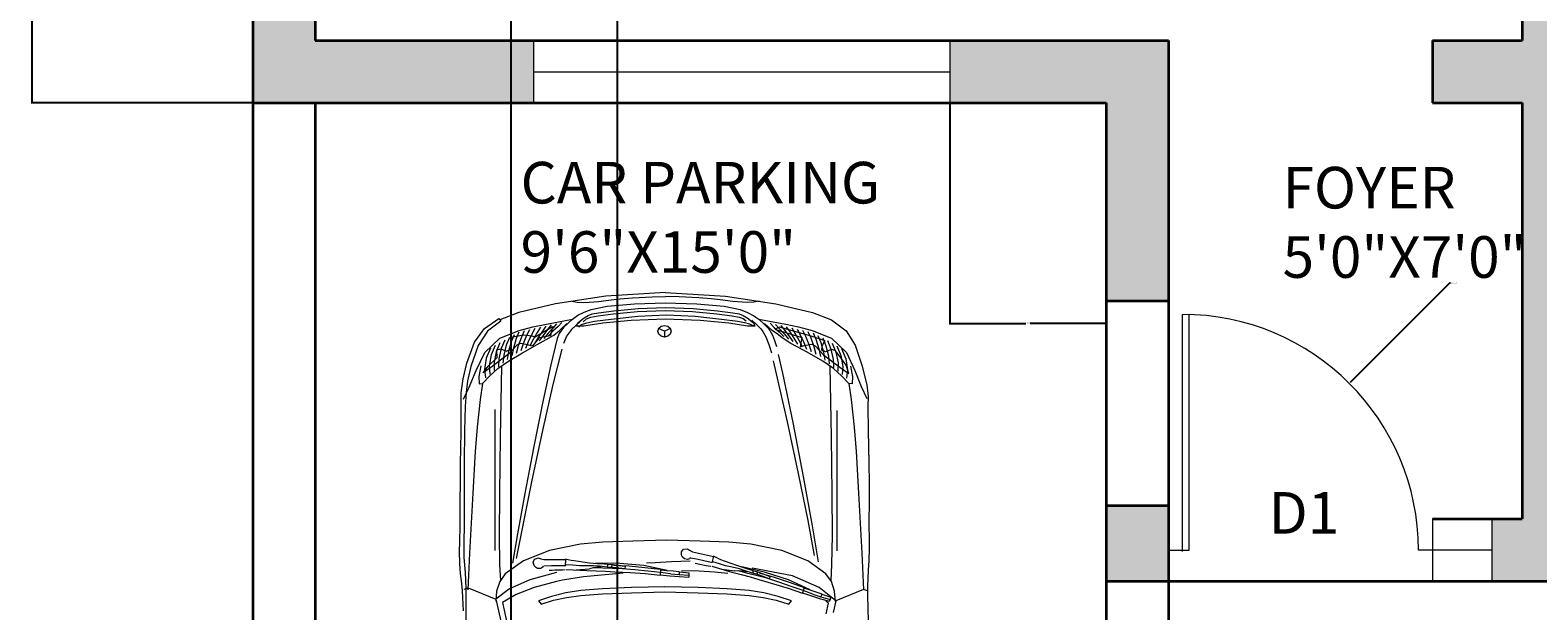
# Model space of a CAD drawing. Units: inches. Extents: x 5 to 421, y -617 to 43.
# Tile 5 of 15: x 5 to 223, y -469 to -385. Entities that reach past the tile are written whole.
import ezdxf

# ---------------------------------------------------------------- set-up
doc = ezdxf.new("R2010")
doc.units = ezdxf.units.IN
doc.header["$MEASUREMENT"] = 0
for name, color, linetype, lineweight in [('A-ANNO-DIMS', 2, 'Continuous', 18), ('A-ANNO-TEXT', 7, 'Continuous', 18), ('A-AREA-IDEN', 7, 'Continuous', 25), ('A-DOOR', 4, 'Continuous', 20), ('A-GLAZ', 4, 'Continuous', 18), ('A-SITE-VEHC', 8, 'Continuous', 13), ('A-WALL', 7, 'Continuous', 35)]:
    doc.layers.add(name, color=color, linetype=linetype, lineweight=lineweight)
doc.layers.add('A-WALL-PATT', color=251, linetype='Continuous', lineweight=13, true_color=0x636466)
doc.styles.get("Standard").update_dxf_attribs({"font": 'arial.ttf'})
doc.dimstyles.get("Standard").update_dxf_attribs({"dimtxt": 0.18, "dimasz": 0.18, "dimexe": 0.18, "dimexo": 0.0625, "dimgap": 0.09, "dimtad": 0, "dimtih": 1, "dimtoh": 1, "dimdec": 0, "dimzin": 0, "dimdsep": 46, "dimlunit": 3, "dimtxsty": 'Standard', "dimcen": 0.09, "dimadec": 0, "dimazin": 0, "dimtfac": 1, "dimtdec": 0, "dimtofl": 0, "dimtmove": 0, "dimatfit": 3, "dimfxl": 1, "dimtolj": 1, "dimtzin": 0, "dimarcsym": 0})

# ---------------------------------------------------------------- blocks, each defined once
blk = doc.blocks.new('WINDOW-W1-60')
for p, q in [((0, 9), (60, 9)), ((0, 0), (0, 9)), ((60, 9), (60, 0)), ((0, 4.5), (60, 4.5)), ((60, 0), (0, 0))]:
    blk.add_line(p, q)
blk = doc.blocks.new('*D55')
at = {"layer": 'A-ANNO-DIMS', "color": 0, "lineweight": -2, "transparency": 16777216}
for p, q in [((370.48, 10.88), (420.4, 10.88)), ((420.22, 10.7), (420.22, -286.69)), ((420.22, -584.44), (420.22, -287.05)), ((169.48, -584.62), (420.4, -584.62))]:
    blk.add_line(p, q, dxfattribs=at)
at = {"layer": 'A-ANNO-DIMS', "color": 0, "transparency": 16777216}
for points in [[(420.19, 10.7), (420.25, 10.7), (420.22, 10.88)], [(420.19, -584.44), (420.25, -584.44), (420.22, -584.62)]]:
    blk.add_solid(points, dxfattribs=at)
at = {"layer": 'Defpoints', "color": 0, "transparency": 16777216}
for p in [(370.42, 10.88), (169.42, -584.62), (420.22, -584.62)]:
    blk.add_point(p, dxfattribs=at)
at = {"layer": 'A-ANNO-DIMS', "color": 0, "transparency": 16777216, "insert": (420.22, -286.87), "char_height": 0.18, "attachment_point": 5}
blk.add_mtext('\\A1;595.5', dxfattribs=at)
blk = doc.blocks.new('*D63')
at = {"layer": 'A-ANNO-DIMS', "color": 0, "lineweight": -2, "transparency": 16777216}
for p, q in [((37.36, -352.8), (5.44, -352.8)), ((5.62, -352.98), (5.62, -374.03)), ((5.62, -395.44), (5.62, -374.39)), ((37.36, -395.62), (5.44, -395.62))]:
    blk.add_line(p, q, dxfattribs=at)
at = {"layer": 'A-ANNO-DIMS', "color": 0, "transparency": 16777216}
for points in [[(5.59, -352.98), (5.65, -352.98), (5.62, -352.8)], [(5.59, -395.44), (5.65, -395.44), (5.62, -395.62)]]:
    blk.add_solid(points, dxfattribs=at)
at = {"layer": 'Defpoints', "color": 0, "transparency": 16777216}
for p in [(37.42, -352.8), (5.62, -395.62), (37.42, -395.62)]:
    blk.add_point(p, dxfattribs=at)
at = {"layer": 'A-ANNO-DIMS', "color": 0, "transparency": 16777216, "insert": (5.62, -374.21), "char_height": 0.18, "attachment_point": 5}
blk.add_mtext('\\A1;42.82', dxfattribs=at)
blk = doc.blocks.new('*D74')
at = {"layer": 'A-ANNO-DIMS', "color": 0, "lineweight": -2, "transparency": 16777216}
for p, q in [((137.92, -395.68), (137.92, -427.6)), ((160.42, -395.68), (160.42, -427.6)), ((138.1, -427.42), (148.84, -427.42)), ((160.24, -427.42), (149.5, -427.42))]:
    blk.add_line(p, q, dxfattribs=at)
at = {"layer": 'A-ANNO-DIMS', "color": 0, "transparency": 16777216}
for points in [[(138.1, -427.39), (138.1, -427.45), (137.92, -427.42)], [(160.24, -427.39), (160.24, -427.45), (160.42, -427.42)]]:
    blk.add_solid(points, dxfattribs=at)
at = {"layer": 'Defpoints', "color": 0, "transparency": 16777216}
for p in [(137.92, -395.62), (160.42, -395.62), (137.92, -427.42)]:
    blk.add_point(p, dxfattribs=at)
at = {"layer": 'A-ANNO-DIMS', "color": 0, "transparency": 16777216, "insert": (149.17, -427.42), "char_height": 0.18, "attachment_point": 5}
blk.add_mtext('\\A1;22.5', dxfattribs=at)
blk = doc.blocks.new('*D78')
at = {"layer": 'A-ANNO-DIMS', "color": 0, "lineweight": -2, "transparency": 16777216}
for p, q in [((74.62, -338.19), (74.62, -616.6)), ((89.92, -338.33), (89.92, -616.6)), ((74.8, -616.42), (81.96, -616.42)), ((89.74, -616.42), (82.59, -616.42))]:
    blk.add_line(p, q, dxfattribs=at)
at = {"layer": 'A-ANNO-DIMS', "color": 0, "transparency": 16777216}
for points in [[(74.8, -616.39), (74.8, -616.45), (74.62, -616.42)], [(89.74, -616.39), (89.74, -616.45), (89.92, -616.42)]]:
    blk.add_solid(points, dxfattribs=at)
at = {"layer": 'Defpoints', "color": 0, "transparency": 16777216}
for p in [(74.62, -338.13), (89.92, -338.27), (89.92, -616.42)]:
    blk.add_point(p, dxfattribs=at)
at = {"layer": 'A-ANNO-DIMS', "color": 0, "transparency": 16777216, "insert": (82.27, -616.42), "char_height": 0.18, "attachment_point": 5}
blk.add_mtext('\\A1;15.3', dxfattribs=at)
blk = doc.blocks.new('*D80')
at = {"layer": 'A-ANNO-DIMS', "color": 0, "lineweight": -2, "transparency": 16777216}
for p, q in [((209.91, -421.62), (195.6, -435.95)), ((210.09, -421.62), (209.91, -421.62)), ((171.33, -460.16), (171.51, -460.16)), ((171.42, -460.25), (171.42, -460.07))]:
    blk.add_line(p, q, dxfattribs=at)
at = {"layer": 'A-ANNO-DIMS', "color": 0, "transparency": 16777216}
blk.add_solid([(195.58, -435.93), (195.63, -435.97), (195.48, -436.07)], dxfattribs=at)
at = {"layer": 'Defpoints', "color": 0, "transparency": 16777216}
for p in [(195.48, -436.07), (171.42, -460.16)]:
    blk.add_point(p, dxfattribs=at)
at = {"layer": 'A-ANNO-DIMS', "color": 0, "transparency": 16777216, "insert": (210.64, -421.62), "char_height": 0.18, "attachment_point": 5}
blk.add_mtext('\\A1;R34.045', dxfattribs=at)

msp = doc.modelspace()

# ---------------------------------------------------------------- hatches: boundary and pattern name
at = {"layer": 'A-WALL-PATT'}
h = msp.add_hatch(color=256, dxfattribs=at)
h.dxf.hatch_style = 1
h.paths.add_polyline_path([(46.4196, -88.1188), (37.4196, -88.1188), (37.4196, -166.6119), (46.4196, -166.6119), (46.4196, -122.6188), (135.4196, -122.6188), (135.4196, -120.3688), (135.4196, -118.1188), (46.4196, -118.1188)])
h.paths.add_polyline_path([(82.4196, 10.8812), (37.4196, 10.8812), (37.4196, -28.1188), (46.4196, -28.1188), (46.4196, 1.8812), (82.4196, 1.8812)])
h.paths.add_polyline_path([(215.5968, 10.8812), (142.4196, 10.8812), (142.4196, 1.8812), (178.4196, 1.8812), (178.4196, -118.1188), (175.4196, -118.1188), (175.4196, -122.6188), (182.9196, -122.6188), (182.9196, -80.6188), (211.9196, -80.6188), (211.9196, -78.3688), (211.9196, -76.1188), (182.9196, -76.1188), (182.9196, 1.8812), (215.5968, 1.8812)])
h.paths.add_polyline_path([(274.4196, 10.8812), (239.5968, 10.8812), (239.5968, 1.8812), (242.9196, 1.8812), (242.9196, -76.1188), (239.9196, -76.1188), (239.9196, -80.6188), (242.9196, -80.6188), (242.9196, -83.6188), (247.4196, -83.6188), (247.4196, 1.8812), (274.4196, 1.8812)])
h.paths.add_polyline_path([(370.4196, 10.8812), (334.4196, 10.8812), (334.4196, 1.8812), (361.4196, 1.8812), (361.4196, -28.1188), (370.4196, -28.1188)])
h.paths.add_polyline_path([(370.4196, -88.1188), (361.4196, -88.1188), (361.4196, -118.1188), (247.4196, -118.1188), (247.4196, -115.1188), (242.9196, -115.1188), (242.9196, -118.1188), (220.4196, -118.1188), (220.4196, -158.6188), (224.9196, -158.6188), (224.9196, -122.6188), (326.9196, -122.6188), (326.9196, -170.7662), (331.4196, -170.7662), (331.4196, -122.6188), (370.4196, -122.6188)])
h.paths.add_polyline_path([(388.4196, -122.6188), (388.4196, -118.1188), (379.4196, -118.1188), (379.4196, -122.6188), (379.4196, -154.8688), (388.4196, -154.8688)])
h.paths.add_polyline_path([(388.4196, -214.8688), (379.4196, -214.8688), (379.4196, -247.1188), (388.4196, -247.1188)])
h.paths.add_polyline_path([(371.0265, -242.6188), (331.4196, -242.6188), (331.4196, -239.6188), (326.9196, -239.6188), (326.9196, -242.6188), (224.9196, -242.6188), (224.9196, -206.6188), (220.4196, -206.6188), (220.4196, -343.6188), (224.9196, -343.6188), (229.4196, -343.6188), (229.4196, -247.1188), (261.5265, -247.1188), (261.5265, -276.1188), (263.7765, -276.1188), (266.0265, -276.1188), (266.0265, -247.1188), (362.0265, -247.1188), (362.0265, -265.1188), (371.0265, -265.1188), (371.0265, -247.1188)])
h.paths.add_polyline_path([(371.0265, -289.1188), (362.0265, -289.1188), (362.0265, -307.1188), (266.0265, -307.1188), (266.0265, -304.1188), (261.5265, -304.1188), (261.5265, -307.1188), (261.5265, -311.6188), (362.0265, -311.6188), (362.0265, -353.6188), (371.0265, -353.6188)])
h.paths.add_polyline_path([(371.0265, -413.6188), (362.0265, -413.6188), (362.0265, -455.6188), (325.7231, -455.6188), (325.7231, -464.6188), (361.4196, -464.6188), (371.0265, -464.6188)])
h.paths.add_polyline_path([(265.7231, -455.6188), (229.4196, -455.6188), (229.4196, -383.6188), (220.4196, -383.6188), (220.4196, -386.6188), (207.4649, -386.6188), (207.4649, -395.6188), (220.4196, -395.6188), (220.4196, -455.6188), (216.0568, -455.6188), (216.0568, -464.6188), (265.7231, -464.6188)])
h.paths.add_polyline_path([(169.4196, -386.6188), (137.9196, -386.6188), (137.9196, -395.6188), (160.4196, -395.6188), (160.4196, -424.2032), (169.4196, -424.2032)])
h.paths.add_polyline_path([(169.4196, -453.7423), (160.4196, -453.7423), (160.4196, -464.6188), (169.4196, -464.6188)])
h.paths.add_polyline_path([(46.4196, -575.6188), (37.4196, -575.6188), (37.4196, -584.6188), (46.4196, -584.6188)])
h.paths.add_polyline_path([(169.4196, -575.6188), (160.4196, -575.6188), (160.4196, -579.5504), (160.4196, -584.6188), (169.4196, -584.6188)])
h.paths.add_polyline_path([(46.4196, -226.6119), (37.4196, -226.6119), (37.4196, -292.8008), (46.4196, -292.8008)])
h.paths.add_polyline_path([(46.4196, -352.8008), (37.4196, -352.8008), (37.4196, -395.6188), (77.9196, -395.6188), (77.9196, -386.6188), (46.4196, -386.6188)])

# ---------------------------------------------------------------- linework, layer by layer
at = {"layer": 'A-DOOR'}
for p, q in [((171.4196, -460.1188), (171.4196, -426.1188)), ((172.4196, -460.1188), (172.4196, -426.1188)), ((207.4649, -455.6188), (207.4649, -464.6188)), ((169.4196, -460.1188), (172.4196, -460.1188)), ((207.4649, -460.1188), (205.4649, -460.1188))]:
    msp.add_line(p, q, dxfattribs=at)
msp.add_arc((171.4196, -460.1641), 34.0453, 0.076254, 90, dxfattribs=at)
at = {"layer": 'A-GLAZ'}
for p, q in [((216.0568, -455.6188), (216.0568, -464.6188)), ((216.0568, -460.1188), (207.4649, -460.1188))]:
    msp.add_line(p, q, dxfattribs=at)
at = {"layer": 'A-SITE-VEHC'}
for p, q in [((88.2888, -423.4807), (81.054, -424.5837)), ((96.9277, -422.9659), (88.2888, -423.4807)), ((90.3721, -423.8704), (92.147, -423.7322)), ((92.147, -423.7322), (94.9644, -423.5941)), ((94.9644, -423.5941), (96.9277, -423.5314)), ((96.9277, -422.9659), (105.5667, -423.4807)), ((98.8913, -423.5941), (96.9277, -423.5314)), ((101.7086, -423.7322), (98.8913, -423.5941)), ((103.4836, -423.8704), (101.7086, -423.7322)), ((105.5667, -423.4807), (112.8017, -424.5837)), ((75.7796, -425.8668), (73.0219, -426.9221)), ((81.054, -424.5837), (75.7796, -425.8668)), ((83.4206, -424.2094), (84.1909, -424.3664)), ((84.1909, -424.3664), (85.0994, -424.4103)), ((84.2586, -426.238), (85.1677, -425.8108)), ((85.0994, -424.4103), (85.9073, -424.3788)), ((85.1677, -425.8108), (86.19, -425.3963)), ((85.9073, -424.3788), (87.228, -424.2471)), ((86.19, -425.3963), (88.484, -424.9461)), ((86.3168, -426.0614), (87.2637, -425.9046)), ((87.228, -424.2471), (89.0889, -424.0399)), ((87.2637, -425.9046), (89.4679, -425.6243)), ((88.484, -424.9461), (92.4484, -424.584)), ((89.0889, -424.0399), (90.3721, -423.8704)), ((89.3807, -426.0595), (92.8658, -425.7162)), ((89.4679, -425.6243), (92.9529, -425.281)), ((92.4484, -424.584), (96.9277, -424.4355)), ((92.8658, -425.7162), (96.8408, -425.5487)), ((92.9529, -425.281), (96.9277, -425.1136)), ((96.8408, -425.5487), (100.8158, -425.7162)), ((96.9277, -424.4355), (101.4072, -424.584)), ((96.9277, -425.1136), (100.9027, -425.281)), ((100.8158, -425.7162), (104.3009, -426.0595)), ((100.9027, -425.281), (104.3878, -425.6243)), ((101.4072, -424.584), (105.3717, -424.9461)), ((104.7667, -424.0399), (103.4836, -423.8704)), ((104.3878, -425.6243), (106.592, -425.9046)), ((106.6275, -424.2471), (104.7667, -424.0399)), ((105.3717, -424.9461), (107.6657, -425.3963)), ((106.592, -425.9046), (107.5389, -426.0614)), ((107.9481, -424.3788), (106.6275, -424.2471)), ((107.6657, -425.3963), (108.7179, -425.8544)), ((108.7562, -424.4103), (107.9481, -424.3788)), ((108.7179, -425.8544), (109.6569, -426.325)), ((109.6648, -424.3664), (108.7562, -424.4103)), ((110.4351, -424.2094), (109.6648, -424.3664)), ((112.8017, -424.5837), (118.0761, -425.8668)), ((118.0761, -425.8668), (120.8338, -426.9221)), ((69.3711, -430.1379), (70.8148, -428.1461)), ((70.8148, -428.1461), (72.9016, -426.7215)), ((73.177, -427.1185), (71.256, -428.5348)), ((72.9016, -426.7215), (73.177, -427.1185)), ((75.7932, -428.4396), (77.7692, -427.9392)), ((78.0926, -428.1602), (77.642, -428.9679)), ((77.7692, -427.9392), (79.7514, -427.5207)), ((78.0971, -429.3429), (80.6258, -427.874)), ((78.8694, -427.9893), (78.4005, -428.7497)), ((79.6462, -427.8179), (79.1591, -428.5313)), ((79.7514, -427.5207), (82.2485, -427.0394)), ((80.4227, -427.6467), (79.9176, -428.313)), ((80.6762, -428.0946), (79.9739, -428.8381)), ((80.6258, -427.874), (80.3167, -429.2124)), ((81.1994, -427.4754), (80.6762, -428.0946)), ((81.4347, -427.8765), (80.6882, -428.5311)), ((81.9759, -427.3041), (81.4347, -427.8765)), ((82.2242, -428.0064), (81.591, -428.8858)), ((81.6239, -428.4674), (82.6858, -427.4308)), ((83.4772, -426.8091), (82.2242, -428.0064)), ((82.2485, -427.0394), (83.4772, -426.8091)), ((84.6587, -427.1007), (83.3473, -428.2992)), ((83.4772, -426.8091), (84.2586, -426.238)), ((84.0633, -427.8201), (84.2663, -427.324)), ((85.1161, -427.8262), (84.0633, -427.8201)), ((84.2663, -427.324), (85.1728, -426.6394)), ((84.4199, -427.9596), (84.8137, -427.5957)), ((84.8137, -427.5957), (85.5658, -427.3175)), ((85.0283, -427.1794), (85.4994, -426.7674)), ((87.8536, -427.4118), (85.1161, -427.8262)), ((85.1728, -426.6394), (85.7717, -426.2683)), ((85.4994, -426.7674), (86.1435, -426.5169)), ((85.5658, -427.3175), (86.6818, -427.1141)), ((85.7717, -426.2683), (86.3168, -426.0614)), ((86.1435, -426.5169), (87.1768, -426.3398)), ((86.6818, -427.1141), (89.0706, -426.8021)), ((87.1768, -426.3398), (89.3807, -426.0595)), ((91.9601, -426.9974), (87.8536, -427.4118)), ((89.0706, -426.8021), (92.8988, -426.4005)), ((96.8713, -426.8091), (91.9601, -426.9974)), ((92.8988, -426.4005), (97.0582, -426.2017)), ((95.8093, -428.5451), (95.9396, -428.1204)), ((96.7635, -428.5451), (95.908, -428.1803)), ((95.9396, -428.1204), (96.2818, -427.8187)), ((96.2818, -427.8187), (96.7635, -427.704)), ((96.7635, -427.704), (97.2447, -427.8187)), ((97.6185, -428.1803), (96.7635, -428.5451)), ((101.9075, -426.9974), (96.8713, -426.8091)), ((97.0582, -426.2017), (101.1968, -426.4005)), ((97.2447, -427.8187), (97.587, -428.1204)), ((97.587, -428.1204), (97.7172, -428.5451)), ((101.1968, -426.4005), (104.9857, -426.8021)), ((106.0206, -427.4118), (101.9075, -426.9974)), ((104.3009, -426.0595), (106.505, -426.3398)), ((104.9857, -426.8021), (107.3534, -427.1141)), ((108.7396, -427.8262), (106.0206, -427.4118)), ((106.505, -426.3398), (107.5061, -426.5108)), ((107.3534, -427.1141), (108.3197, -427.2686)), ((107.5061, -426.5108), (108.1116, -426.7281)), ((107.5389, -426.0614), (108.084, -426.2683)), ((108.084, -426.2683), (108.6829, -426.6394)), ((108.1116, -426.7281), (108.5549, -427.0488)), ((108.3197, -427.2686), (108.9991, -427.4664)), ((108.6829, -426.6394), (109.5893, -427.324)), ((109.7923, -427.8201), (108.7396, -427.8262)), ((108.9991, -427.4664), (109.5727, -427.767)), ((109.3336, -426.9632), (110.1205, -427.6759)), ((109.5893, -427.324), (109.7923, -427.8201)), ((109.6569, -426.325), (110.3785, -426.8091)), ((110.1205, -427.6759), (110.6529, -428.1921)), ((110.3785, -426.8091), (111.1529, -427.5355)), ((110.3785, -426.8091), (111.9209, -427.0823)), ((110.6529, -428.1921), (110.9445, -428.5744)), ((111.1529, -427.5355), (111.6762, -428.0607)), ((112.3063, -428.4628), (111.1699, -427.4308)), ((111.6762, -428.0607), (111.9609, -428.448)), ((111.9209, -427.0823), (114.2611, -427.5423)), ((111.9928, -427.3914), (112.5341, -427.9635)), ((112.5341, -427.9635), (113.2805, -428.6182)), ((113.3429, -427.9612), (112.6534, -428.2674)), ((112.7696, -427.5623), (113.2927, -428.1817)), ((113.2927, -428.1817), (113.9949, -428.9252)), ((116.2301, -428.8039), (113.3429, -427.9612)), ((113.5461, -427.7336), (114.0511, -428.4001)), ((114.2611, -427.5423), (116.0865, -427.9392)), ((114.3225, -427.9048), (114.8095, -428.6184)), ((115.0993, -428.0761), (115.5682, -428.8366)), ((116.0865, -427.9392), (118.0625, -428.4396)), ((120.8338, -426.9221), (122.9445, -428.4988)), ((68.2734, -433.1631), (69.3711, -430.1379)), ((71.256, -428.5348), (69.9184, -430.6081)), ((70.8743, -431.6128), (73.0385, -429.5678)), ((73.0423, -430.2084), (72.5012, -431.5059)), ((73.0385, -429.5678), (75.7932, -428.4396)), ((73.7226, -429.8248), (73.2176, -431.0352)), ((74.4026, -429.4412), (73.9338, -430.5644)), ((74.65, -430.0936), (74.2772, -431.4987)), ((74.6156, -429.4297), (76.4147, -429.0668)), ((74.639, -429.7757), (74.6156, -429.4297)), ((74.6409, -430.5092), (74.639, -429.7757)), ((75.0826, -429.0576), (74.65, -430.0936)), ((75.3663, -429.6228), (74.9727, -430.9883)), ((75.7626, -428.674), (75.3663, -429.6228)), ((75.9564, -430.3259), (75.464, -430.557)), ((76.1248, -429.4047), (75.6872, -430.6813)), ((77.0534, -430.5351), (75.9564, -430.3259)), ((76.539, -428.5027), (76.1248, -429.4047)), ((76.8835, -429.1863), (76.4017, -430.3741)), ((76.4147, -429.0668), (77.6427, -429.1952)), ((77.1161, -430.0668), (76.71, -431.0374)), ((77.3162, -428.3315), (76.8835, -429.1863)), ((77.642, -428.9679), (77.1161, -430.0668)), ((77.8305, -429.7597), (77.3697, -430.6786)), ((77.6427, -429.1952), (78.0971, -429.3429)), ((78.7064, -429.517), (77.6619, -430.7102)), ((78.4005, -428.7497), (77.8305, -429.7597)), ((78.5449, -429.4525), (78.0296, -430.3192)), ((78.4145, -430.4721), (80.1428, -429.5218)), ((79.1591, -428.5313), (78.5449, -429.4525)), ((79.2594, -429.1454), (78.6892, -429.9604)), ((80.3167, -429.2124), (78.7064, -429.517)), ((79.9176, -428.313), (79.2594, -429.1454)), ((79.9739, -428.8381), (79.3491, -429.6011)), ((80.6882, -428.5311), (80.0088, -429.2423)), ((80.1428, -429.5218), (80.8255, -429.102)), ((81.3112, -429.596), (80.3544, -433.4005)), ((80.8255, -429.102), (81.6239, -428.4674)), ((81.591, -428.8858), (81.3112, -429.596)), ((82.3299, -429.9862), (82.2169, -430.333)), ((82.6517, -429.2407), (82.3299, -429.9862)), ((83.3473, -428.2992), (82.6517, -429.2407)), ((95.9396, -428.9696), (95.8093, -428.5451)), ((96.2818, -429.2716), (95.9396, -428.9696)), ((96.7635, -429.3865), (96.2818, -429.2716)), ((96.7635, -428.5451), (96.7635, -429.3865)), ((97.2447, -429.2716), (96.7635, -429.3865)), ((97.587, -428.9696), (97.2447, -429.2716)), ((97.7172, -428.5451), (97.587, -428.9696)), ((110.9445, -428.5744), (111.3801, -429.3839)), ((111.3801, -429.3839), (111.8254, -430.4731)), ((111.9609, -428.448), (112.3202, -429.1271)), ((113.1791, -429.0928), (112.3063, -428.4628)), ((112.3202, -429.1271), (112.6292, -429.9037)), ((112.6292, -429.9037), (112.8982, -430.7589)), ((112.6534, -428.2674), (116.5621, -429.4677)), ((113.7129, -429.5218), (113.1791, -429.0928)), ((113.2805, -428.6182), (113.9599, -429.3291)), ((114.9855, -430.311), (113.7129, -429.5218)), ((113.9949, -428.9252), (114.6195, -429.6882)), ((114.0511, -428.4001), (114.7092, -429.2325)), ((114.7092, -429.2325), (115.2792, -430.0474)), ((114.8095, -428.6184), (115.4237, -429.5396)), ((117.3382, -431.5773), (114.9855, -430.311)), ((115.4237, -429.5396), (115.9391, -430.4065)), ((115.5682, -428.8366), (116.1383, -429.8467)), ((115.8761, -428.2474), (116.3267, -429.055)), ((116.1383, -429.8467), (116.5991, -430.7656)), ((116.7357, -428.9249), (116.2301, -428.8039)), ((116.5621, -429.4677), (116.3069, -430.7974)), ((116.3267, -429.055), (116.8525, -430.1539)), ((116.6525, -428.4187), (117.0852, -429.2733)), ((118.0587, -429.2957), (116.7357, -428.9249)), ((116.8525, -430.1539), (117.2587, -431.1247)), ((117.0852, -429.2733), (117.5669, -430.461)), ((117.4293, -428.59), (117.8439, -429.4917)), ((117.8439, -429.4917), (118.2815, -430.7682)), ((119.909, -429.9274), (118.0587, -429.2957)), ((118.0625, -428.4396), (120.8172, -429.5678)), ((118.2061, -428.7609), (118.6025, -429.7099)), ((118.6025, -429.7099), (118.996, -431.0754)), ((118.8861, -429.1445), (119.3186, -430.1807)), ((119.3186, -430.1807), (119.6916, -431.5858)), ((119.4719, -430.7027), (119.7415, -430.1668)), ((119.5662, -429.5281), (120.0349, -430.6515)), ((119.7415, -430.1668), (119.909, -429.9274)), ((120.2461, -429.9118), (120.751, -431.1223)), ((120.8172, -429.5678), (122.9814, -431.6128)), ((120.9262, -430.2954), (121.4674, -431.5931)), ((122.9445, -428.4988), (124.2439, -430.5614)), ((69.9184, -430.6081), (68.8652, -433.6607)), ((69.6163, -434.2354), (70.8743, -431.6128)), ((71.0689, -432.4475), (70.7995, -434.0515)), ((71.6826, -430.9754), (71.0689, -432.4475)), ((71.3212, -433.5838), (72.65, -432.3556)), ((71.7852, -431.9768), (71.495, -433.541)), ((72.3626, -430.592), (71.7852, -431.9768)), ((74.2891, -431.8677), (71.9248, -433.6635)), ((72.5012, -431.5059), (72.1905, -433.0304)), ((72.608, -431.2511), (73.1494, -431.1126)), ((72.65, -432.3556), (72.608, -431.2511)), ((72.8862, -432.5199), (72.8414, -433.683)), ((73.2176, -431.0352), (72.8862, -432.5199)), ((73.1494, -431.1126), (73.9886, -431.4394)), ((73.5817, -432.0093), (73.4711, -433.1602)), ((73.9338, -430.5644), (73.5817, -432.0093)), ((73.9886, -431.4394), (74.5191, -431.174)), ((74.2772, -431.4987), (74.1008, -432.6375)), ((74.265, -432.8562), (76.2895, -431.658)), ((75.464, -430.557), (74.2891, -431.8677)), ((74.5191, -431.174), (74.6409, -430.5092)), ((74.9727, -430.9883), (74.7305, -432.1151)), ((75.6872, -430.6813), (75.3905, -431.756)), ((76.4017, -430.3741), (76.0504, -431.3969)), ((76.2895, -431.658), (78.4145, -430.4721)), ((77.6619, -430.7102), (77.0534, -430.5351)), ((81.9727, -431.1396), (80.6692, -436.2199)), ((111.8254, -430.4731), (112.1838, -431.6837)), ((113.1414, -431.9011), (113.3375, -432.7409)), ((116.3069, -430.7974), (116.9153, -430.6223)), ((116.9153, -430.6223), (118.0123, -430.4132)), ((119.5903, -432.8562), (117.3382, -431.5773)), ((117.5669, -430.461), (117.9184, -431.4838)), ((118.0123, -430.4132), (118.5048, -430.6443)), ((118.2815, -430.7682), (118.5783, -431.8429)), ((118.5048, -430.6443), (119.6796, -431.9549)), ((118.996, -431.0754), (119.2379, -432.202)), ((119.4496, -431.2613), (119.4719, -430.7027)), ((119.9802, -431.5265), (119.4496, -431.2613)), ((119.6796, -431.9549), (122.0438, -433.7505)), ((119.6916, -431.5858), (119.8679, -432.7248)), ((120.8193, -431.1998), (119.9802, -431.5265)), ((120.0349, -430.6515), (120.3871, -432.0964)), ((120.3871, -432.0964), (120.4976, -433.2471)), ((120.751, -431.1223), (121.0826, -432.607)), ((121.3607, -431.3383), (120.8193, -431.1998)), ((121.9401, -432.0338), (121.3607, -431.3383)), ((121.4674, -431.5931), (121.7781, -433.1176)), ((121.6061, -430.679), (122.1836, -432.0637)), ((122.9582, -433.4664), (121.9401, -432.0338)), ((122.1836, -432.0637), (122.4737, -433.628)), ((122.2864, -431.0626), (122.8999, -432.5347)), ((122.8999, -432.5347), (123.1693, -434.1386)), ((122.9814, -431.6128), (124.2013, -434.2101)), ((124.2439, -430.5614), (125.2421, -433.591)), ((67.7369, -435.4045), (68.2734, -433.1631)), ((68.8652, -433.6607), (68.3838, -435.6874)), ((68.6094, -436.6196), (69.6163, -434.2354)), ((70.2847, -433.5477), (69.979, -435.0678)), ((70.6339, -434.568), (71.3212, -433.5838)), ((71.9248, -433.6635), (70.6339, -434.568)), ((70.7995, -434.0515), (70.952, -435.2509)), ((71.495, -433.541), (71.5816, -434.7281)), ((71.5776, -434.9912), (72.733, -433.9426)), ((72.1905, -433.0304), (72.2117, -434.2057)), ((72.733, -433.9426), (74.265, -432.8562)), ((73.248, -433.591), (73.0571, -443.8216)), ((80.3544, -433.4005), (79.1612, -438.9485)), ((112.4369, -432.8317), (112.5824, -433.454)), ((112.5824, -433.454), (112.7269, -434.0792)), ((112.7269, -434.0792), (112.8734, -434.7023)), ((112.8734, -434.7023), (114.4492, -441.6229)), ((113.3375, -432.7409), (113.5855, -433.768)), ((113.5855, -433.768), (113.7826, -434.6088)), ((113.7826, -434.6088), (115.2521, -441.7013)), ((121.1226, -433.9426), (119.5903, -432.8562)), ((120.6077, -433.591), (120.7986, -443.8216)), ((121.0826, -432.607), (121.1273, -433.7699)), ((122.278, -434.9912), (121.1226, -433.9426)), ((121.7781, -433.1176), (121.7573, -434.2926)), ((122.0438, -433.7505), (123.3348, -434.6549)), ((122.4737, -433.628), (122.387, -434.8154)), ((123.3348, -434.6549), (122.9582, -433.4664)), ((123.1693, -434.1386), (123.0168, -435.3377)), ((123.5863, -433.6012), (123.8799, -435.1001)), ((124.2013, -434.2101), (125.1374, -436.5473)), ((125.2421, -433.591), (125.9265, -436.3435)), ((67.4732, -437.448), (67.7369, -435.4045)), ((67.7659, -438.3383), (68.6094, -436.6196)), ((68.3838, -435.6874), (68.1627, -437.3774)), ((69.979, -435.0678), (70.0263, -436.1261)), ((70.0263, -436.1261), (70.5352, -436.0776)), ((70.5352, -436.0776), (70.1814, -438.4136)), ((70.5352, -436.0776), (71.5776, -434.9912)), ((80.6692, -436.2199), (79.1628, -442.8862)), ((123.3205, -436.0776), (122.278, -434.9912)), ((123.3205, -436.0776), (123.6742, -438.4136)), ((123.8264, -436.1331), (123.3205, -436.0776)), ((123.8799, -435.1001), (123.8264, -436.1331)), ((125.1374, -436.5473), (125.9431, -438.2405)), ((125.9265, -436.3435), (126.1212, -437.9406)), ((67.4465, -439.6913), (67.4732, -437.448)), ((68.1627, -437.3774), (68.027, -439.4035)), ((70.1814, -438.4136), (69.7398, -442.3696)), ((79.1612, -438.9485), (77.8734, -445.4109)), ((123.6742, -438.4136), (124.1158, -442.3696)), ((126.1212, -437.9406), (126.0898, -439.412)), ((67.4427, -443.068), (67.4465, -439.6913)), ((68.027, -439.4035), (67.9392, -442.8546)), ((72.3562, -460.1668), (72.3562, -439.8489)), ((121.6428, -460.2288), (121.6428, -439.9915)), ((126.0898, -439.412), (126.1085, -442.8615)), ((67.3766, -447.6771), (67.4427, -443.068)), ((67.9392, -442.8546), (67.8914, -447.602)), ((69.7398, -442.3696), (69.4615, -445.9112)), ((79.1628, -442.8862), (77.6474, -450.0302)), ((114.4492, -441.6229), (116.0351, -449.0681)), ((115.2521, -441.7013), (116.74, -449.4932)), ((124.1158, -442.3696), (124.3942, -445.9112)), ((126.1085, -442.8615), (126.2027, -447.6046)), ((73.0571, -443.8216), (72.9558, -451.9309)), ((77.8734, -445.4109), (76.6326, -451.958)), ((120.7986, -443.8216), (120.8999, -451.9309)), ((67.3351, -450.4891), (67.3766, -447.6771)), ((67.8914, -447.602), (67.877, -450.4891)), ((69.4615, -445.9112), (69.1454, -451.9124)), ((124.3942, -445.9112), (124.7103, -451.9124)), ((126.2027, -447.6046), (126.2592, -450.4891)), ((116.0351, -449.0681), (117.4126, -455.8761)), ((116.74, -449.4932), (118.0308, -456.6443)), ((67.3241, -452.8999), (67.3351, -450.4891)), ((67.877, -450.4891), (67.8795, -452.8906)), ((69.1454, -451.9124), (68.6659, -460.5759)), ((72.9558, -451.9309), (72.9386, -458.0219)), ((76.6326, -451.958), (75.5807, -457.7605)), ((77.6474, -450.0302), (76.3174, -456.5443)), ((120.8999, -451.9309), (120.9171, -458.0219)), ((124.7103, -451.9124), (125.1898, -460.5759)), ((126.2592, -450.4891), (126.2466, -452.8272)), ((67.2929, -456.5931), (67.3241, -452.8999)), ((67.8795, -452.8906), (67.8734, -456.5629)), ((126.2466, -452.8272), (126.2342, -456.3835)), ((117.4126, -455.8761), (118.3637, -460.885)), ((126.2342, -456.3835), (126.2592, -458.6839)), ((67.2441, -458.9666), (67.2929, -456.5931)), ((67.8734, -456.5629), (67.8382, -458.9265)), ((72.9386, -458.0219), (73.0001, -462.1977)), ((75.5807, -457.7605), (74.8595, -461.9887)), ((76.3174, -456.5443), (75.3669, -461.3202)), ((118.0308, -456.6443), (118.9091, -461.8146)), ((120.9171, -458.0219), (120.8556, -462.1977)), ((67.2233, -460.2932), (67.2441, -458.9666)), ((67.266, -462.0552), (67.2233, -460.2932)), ((67.8382, -458.9265), (67.8416, -461.1709)), ((68.6659, -460.5759), (68.3876, -465.8612)), ((80.1909, -460.1741), (76.4305, -461.677)), ((84.6357, -459.249), (80.1909, -460.1741)), ((87.8747, -458.9991), (84.6357, -459.249)), ((92.1991, -458.8343), (87.8747, -458.9991)), ((97.083, -458.7091), (92.1991, -458.8343)), ((101.8865, -458.8343), (97.083, -458.7091)), ((99.1984, -460.7374), (99.2068, -460.3723)), ((99.2698, -460.9719), (99.1984, -460.7374)), ((99.2068, -460.3723), (99.498, -459.9927)), ((99.498, -459.9927), (100.0704, -459.9314)), ((100.0704, -459.9314), (100.3911, -460.1555)), ((100.3911, -460.1555), (100.782, -460.3626)), ((100.782, -460.3626), (103.8287, -461.0493)), ((106.0614, -458.9991), (101.8865, -458.8343)), ((109.22, -459.249), (106.0614, -458.9991)), ((113.6648, -460.1741), (109.22, -459.249)), ((117.4252, -461.677), (113.6648, -460.1741)), ((125.1898, -460.5759), (125.4681, -465.8612)), ((126.2802, -459.9627), (126.2384, -461.6435)), ((126.2592, -458.6839), (126.2802, -459.9627)), ((67.3594, -463.4958), (67.266, -462.0552)), ((67.8416, -461.1709), (68.0069, -463.3588)), ((73.0001, -462.1977), (73.1349, -464.5613)), ((76.4305, -461.677), (73.813, -463.5442)), ((77.8329, -461.8644), (78.0312, -461.4291)), ((77.9068, -462.2219), (77.8329, -461.8644)), ((78.029, -462.4344), (77.9068, -462.2219)), ((78.1517, -462.5649), (78.029, -462.4344)), ((78.0312, -461.4291), (78.575, -461.2407)), ((78.4749, -462.7683), (78.1517, -462.5649)), ((78.9309, -462.7623), (78.4749, -462.7683)), ((78.575, -461.2407), (78.938, -461.3869)), ((79.2105, -462.5944), (78.9309, -462.7623)), ((78.938, -461.3869), (79.3654, -461.5007)), ((79.2344, -462.4904), (79.2105, -462.5944)), ((79.2798, -462.4361), (79.2344, -462.4904)), ((79.3654, -461.5007), (82.4884, -461.4845)), ((80.4498, -462.413), (79.3695, -462.4376)), ((81.2567, -462.4009), (80.4498, -462.413)), ((80.958, -462.9925), (81.3615, -462.9693)), ((82.3369, -462.3848), (81.2567, -462.4009)), ((81.3615, -462.9693), (81.7181, -462.9591)), ((81.7181, -462.9591), (82.075, -462.9503)), ((82.075, -462.9503), (82.4311, -462.9346)), ((82.4932, -461.4342), (82.4365, -462.422)), ((82.8969, -461.5126), (82.4932, -461.4342)), ((82.5744, -462.918), (85.586, -463.0884)), ((83.5508, -462.3194), (82.5767, -462.2555)), ((83.3179, -461.6139), (82.8969, -461.5126)), ((83.7224, -461.6898), (83.3179, -461.6139)), ((84.4899, -462.3828), (83.5508, -462.3194)), ((84.9791, -461.8593), (83.7224, -461.6898)), ((84.0128, -462.9941), (85.962, -462.8056)), ((85.4667, -462.3924), (84.4899, -462.3828)), ((85.9278, -461.986), (84.9791, -461.8593)), ((86.5356, -462.3913), (85.4667, -462.3924)), ((87.102, -462.0849), (85.9278, -461.986)), ((86.512, -462.7033), (85.962, -462.8056)), ((87.8734, -462.7421), (86.4771, -462.7028)), ((87.0621, -462.592), (86.512, -462.7033)), ((87.4029, -462.4626), (86.5356, -462.3913)), ((90.3032, -462.0456), (86.8254, -462.0183)), ((87.6187, -462.5538), (87.0621, -462.592)), ((87.5711, -462.121), (87.102, -462.0849)), ((88.4907, -462.5809), (87.4029, -462.4626)), ((88.0494, -462.1638), (87.5711, -462.121)), ((89.2705, -462.7601), (87.8734, -462.7421)), ((88.5168, -462.1994), (88.0494, -462.1638)), ((88.476, -462.5191), (89.3352, -462.5761)), ((88.5238, -462.2303), (88.4907, -462.5809)), ((89.3664, -462.273), (88.5047, -462.2186)), ((89.1681, -462.2612), (89.1395, -462.5618)), ((90.6673, -462.8136), (89.2705, -462.7601)), ((89.3352, -462.5761), (90.1995, -462.6739)), ((90.2314, -462.3803), (89.3664, -462.273)), ((89.4222, -462.3007), (91.6841, -462.4046)), ((90.1995, -462.6739), (91.0537, -462.7897)), ((91.0859, -462.5045), (90.2314, -462.3803)), ((93.7649, -462.3516), (90.3032, -462.0456)), ((92.5073, -462.9701), (90.6673, -462.8136)), ((91.0859, -462.5045), (91.0381, -462.7932)), ((91.6841, -462.4046), (93.9504, -462.6448)), ((97.1716, -463.0431), (93.7649, -462.3516)), ((93.9504, -462.6448), (96.2053, -462.8903)), ((95.4127, -461.9535), (94.1669, -462.0165)), ((97.7619, -461.8221), (95.4127, -461.9535)), ((96.2053, -462.8903), (96.1601, -463.6849)), ((96.2041, -462.9562), (97.1006, -463.047)), ((100.4863, -461.7401), (97.7619, -461.8221)), ((99.3601, -461.1267), (99.2698, -460.9719)), ((99.6292, -461.3975), (99.3601, -461.1267)), ((100.0749, -461.4943), (99.6292, -461.3975)), ((100.3851, -461.3934), (100.0749, -461.4943)), ((100.4319, -461.2974), (100.3851, -461.3934)), ((100.4884, -461.2546), (100.4319, -461.2974)), ((101.6334, -461.4955), (100.5754, -461.2766)), ((101.2028, -462.0037), (101.8731, -462.1595)), ((102.4223, -461.6652), (101.6334, -461.4955)), ((101.8731, -462.1595), (102.7923, -462.3346)), ((103.4785, -461.8926), (102.4223, -461.6652)), ((102.7923, -462.3346), (103.4466, -462.4494)), ((103.8445, -461.0015), (103.5672, -461.9512)), ((103.5899, -462.4653), (106.4863, -463.309)), ((104.6761, -462.1018), (103.7414, -461.8206)), ((104.325, -461.2219), (103.8445, -461.0015)), ((104.9082, -461.5095), (104.325, -461.2219)), ((105.5769, -462.375), (104.6761, -462.1018)), ((105.395, -461.7118), (104.9082, -461.5095)), ((104.9744, -462.8632), (106.9161, -463.118)), ((106.3639, -462.0388), (105.395, -461.7118)), ((106.5267, -462.6038), (105.5769, -462.375)), ((107.2003, -462.3592), (106.3639, -462.0388)), ((107.5681, -462.8432), (106.5267, -462.6038)), ((108.1891, -462.6722), (107.2003, -462.3592)), ((108.3972, -463.1079), (107.5681, -462.8432)), ((111.3169, -463.354), (107.9344, -462.5449)), ((108.6395, -462.8074), (108.1891, -462.6722)), ((109.0952, -462.9594), (108.6395, -462.8074)), ((109.5418, -463.102), (109.0952, -462.9594)), ((115.2037, -463.8572), (109.3941, -462.7305)), ((120.0427, -463.5442), (117.4252, -461.677)), ((120.8556, -462.1977), (120.7208, -464.5613)), ((126.2384, -461.6435), (126.1465, -463.0355)), ((67.4763, -464.5583), (67.3594, -463.4958)), ((67.5754, -465.4841), (67.4763, -464.5583)), ((68.0069, -463.3588), (68.1046, -465.5979)), ((73.0243, -464.6698), (72.5615, -466.0316)), ((73.813, -463.5442), (73.0243, -464.6698)), ((77.3422, -464.4164), (74.4145, -465.7233)), ((81.1985, -463.3525), (77.3422, -464.4164)), ((81.1985, -464.6581), (77.9846, -465.5056)), ((80.1447, -463.0052), (80.5468, -463.0136)), ((80.5468, -463.0136), (80.958, -462.9925)), ((82.077, -464.4532), (81.1985, -464.6581)), ((85.0885, -463.982), (82.077, -464.4532)), ((90.7968, -463.4595), (85.0885, -463.982)), ((85.586, -463.0884), (86.9306, -463.1005)), ((86.9306, -463.1005), (88.2809, -463.1695)), ((88.2809, -463.1695), (89.625, -463.2501)), ((89.625, -463.2501), (91.7957, -463.3613)), ((91.7957, -463.3613), (93.9995, -463.5079)), ((94.3443, -463.1673), (92.5073, -462.9701)), ((93.9995, -463.5079), (96.1592, -463.7505)), ((96.1818, -463.3532), (94.3443, -463.1673)), ((96.1601, -463.6849), (97.5238, -463.8326)), ((97.6487, -463.5534), (96.1697, -463.3723)), ((97.1006, -463.047), (97.9979, -463.126)), ((97.5238, -463.8326), (98.8844, -463.9397)), ((97.6487, -463.5534), (98.863, -463.649)), ((97.9979, -463.126), (98.8942, -463.2169)), ((98.9012, -463.2481), (98.863, -463.649)), ((98.863, -463.649), (100.2586, -463.7514)), ((98.8844, -463.9397), (100.2539, -464.0137)), ((98.9012, -463.2481), (99.3611, -463.2968)), ((101.7521, -463.1711), (99.2087, -463.1256)), ((99.3611, -463.2968), (99.8221, -463.3543)), ((99.8221, -463.3543), (100.28, -463.4197)), ((100.28, -463.4197), (100.2539, -464.0137)), ((103.9888, -463.302), (101.7521, -463.1711)), ((105.8849, -463.484), (103.9888, -463.302)), ((106.4863, -463.309), (107.7936, -463.6232)), ((107.4751, -463.142), (106.9161, -463.118)), ((108.7927, -463.4861), (107.441, -463.1339)), ((108.036, -463.1573), (107.4751, -463.142)), ((107.7936, -463.6232), (109.0937, -463.9942)), ((108.5867, -463.2452), (108.036, -463.1573)), ((109.4304, -463.4681), (108.3972, -463.1079)), ((110.1499, -463.8178), (108.7927, -463.4861)), ((109.0937, -463.9942), (110.3851, -464.3751)), ((109.5418, -463.1339), (109.4304, -463.4681)), ((109.4304, -463.4045), (110.2545, -463.6532)), ((110.3531, -463.3647), (109.5259, -463.118)), ((110.1623, -463.309), (110.0668, -463.5951)), ((111.4991, -464.1841), (110.1499, -463.8178)), ((110.2545, -463.6532), (111.0745, -463.9428)), ((111.1718, -463.6639), (110.3531, -463.3647)), ((110.3851, -464.3751), (112.4751, -464.9717)), ((110.401, -463.4045), (112.5817, -464.0144)), ((111.0745, -463.9428), (111.881, -464.2478)), ((111.9765, -463.9772), (111.1718, -463.6639)), ((114.6211, -464.4308), (111.3169, -463.354)), ((113.2566, -464.7506), (111.4991, -464.1841)), ((111.9765, -463.9772), (111.8651, -464.2478)), ((112.4751, -464.9717), (114.5894, -465.6104)), ((112.5817, -464.0144), (114.736, -464.7583)), ((115.0022, -465.356), (113.2566, -464.7506)), ((117.7849, -465.8711), (114.6211, -464.4308)), ((114.736, -464.7583), (116.878, -465.5049)), ((119.0541, -465.5246), (115.2037, -463.8572)), ((120.8314, -464.6698), (120.0427, -463.5442)), ((121.2942, -466.0316), (120.8314, -464.6698)), ((126.0542, -464.2139), (126.0123, -465.3798)), ((126.1465, -463.0355), (126.0542, -464.2139)), ((67.6235, -465.9802), (67.5754, -465.4841)), ((67.6725, -466.951), (67.6235, -465.9802)), ((67.7642, -468.9053), (67.6725, -466.951)), ((67.8811, -465.7587), (68.4427, -465.59)), ((68.1046, -465.5979), (68.1241, -465.6435)), ((68.1289, -466.2525), (68.1156, -468.0292)), ((68.1241, -465.6435), (68.1369, -465.6954)), ((68.1422, -465.7536), (68.1289, -466.2525)), ((68.1369, -465.6954), (68.1422, -465.7536)), ((68.4427, -465.59), (72.4317, -467.2193)), ((74.4145, -465.7233), (72.4317, -467.2193)), ((72.4317, -467.2193), (72.8166, -468.888)), ((72.5615, -466.0316), (72.4568, -467.5567)), ((75.386, -466.5216), (73.4116, -467.6765)), ((77.9846, -465.5056), (75.386, -466.5216)), ((80.4929, -466.8018), (78.5908, -467.4339)), ((82.5401, -466.3), (80.4929, -466.8018)), ((80.7806, -467.3647), (82.6408, -466.9781)), ((84.6848, -465.9506), (82.5401, -466.3)), ((82.6408, -466.9781), (84.6848, -466.6908)), ((87.8434, -465.701), (84.6848, -465.9506)), ((84.6848, -466.6908), (87.8434, -466.4409)), ((92.0183, -465.5362), (87.8434, -465.701)), ((87.8434, -466.4409), (92.0183, -466.2759)), ((96.8217, -465.4107), (92.0183, -465.5362)), ((92.0183, -466.2759), (96.8217, -466.1506)), ((101.6251, -465.5362), (96.8217, -465.4107)), ((96.8217, -466.1506), (101.6251, -466.2759)), ((105.8002, -465.701), (101.6251, -465.5362)), ((101.6251, -466.2759), (105.8002, -466.4409)), ((108.9589, -465.9506), (105.8002, -465.701)), ((105.8002, -466.4409), (108.9589, -466.6908)), ((111.1033, -466.3), (108.9589, -465.9506)), ((108.9589, -466.6908), (111.0027, -466.9781)), ((111.0027, -466.9781), (112.863, -467.3647)), ((113.1505, -466.8018), (111.1033, -466.3)), ((115.0529, -467.4339), (113.1505, -466.8018)), ((114.5894, -465.6104), (116.6392, -466.3324)), ((116.7506, -465.9506), (115.0022, -465.356)), ((116.878, -465.5049), (116.6551, -466.269)), ((116.6551, -466.269), (117.9507, -466.7195)), ((118.1351, -466.4756), (116.7347, -465.9666)), ((116.8621, -465.5686), (117.7149, -465.8589)), ((117.7149, -465.8589), (118.5713, -466.1377)), ((117.9507, -466.7195), (119.2522, -467.1298)), ((118.1351, -466.4756), (119.2968, -466.8417)), ((118.5713, -466.1377), (119.4242, -466.4279)), ((121.4807, -467.4597), (119.0541, -465.5246)), ((119.2522, -467.1298), (120.5699, -467.51)), ((119.4242, -466.4597), (119.2968, -466.8417)), ((119.2968, -466.8417), (120.6335, -467.2556)), ((119.4242, -466.4597), (119.8614, -466.6107)), ((119.8614, -466.6107), (120.2975, -466.7705)), ((120.2975, -466.7705), (120.729, -466.9372)), ((120.729, -466.9372), (120.5699, -467.51)), ((121.3989, -467.5567), (121.2942, -466.0316)), ((125.4694, -465.8303), (121.4807, -467.4597)), ((126.0312, -465.9991), (125.4694, -465.8303)), ((126.0123, -465.3798), (126.0332, -466.0308)), ((126.0332, -466.0308), (126.0416, -466.6441)), ((126.0416, -466.6441), (126.0856, -468.6013)), ((68.1156, -468.0292), (68.1428, -471.5036)), ((72.8166, -468.888), (73.6384, -472.4794)), ((73.4116, -467.6765), (76.9484, -483.8294)), ((78.5908, -467.4339), (78.979, -467.935)), ((78.979, -467.935), (80.7806, -467.3647)), ((112.863, -467.3647), (114.6647, -467.935)), ((114.6647, -467.935), (115.0529, -467.4339)), ((120.1486, -467.5806), (120.0128, -467.4937)), ((120.0545, -469.2979), (120.4101, -467.7799)), ((120.2811, -467.6777), (120.1486, -467.5806)), ((120.4101, -467.7799), (120.2811, -467.6777)), ((121.4807, -467.4597), (121.0957, -469.1284)), ((126.0856, -468.6013), (126.1926, -472.0787))]:
    msp.add_line(p, q, dxfattribs=at)
at = {"layer": 'A-WALL'}
for p, q in [((37.4196, 10.8812), (37.4196, -584.6188)), ((46.4196, -122.6188), (46.4196, -386.6188)), ((220.4196, -206.6188), (220.4196, -386.6188)), ((46.4196, -386.6188), (169.4196, -386.6188)), ((169.4196, -386.6188), (169.4196, -584.6188)), ((207.4649, -386.6188), (207.4649, -395.6188)), ((207.4649, -386.6188), (220.4196, -386.6188)), ((37.4196, -395.6188), (160.4196, -395.6188)), ((46.4196, -395.6188), (46.4196, -584.6188)), ((160.4196, -395.6188), (160.4196, -584.6188)), ((207.4649, -395.6188), (220.4196, -395.6188)), ((220.4196, -395.6188), (220.4196, -455.6188)), ((169.4196, -424.2032), (160.4196, -424.2032)), ((169.4196, -453.7423), (160.4196, -453.7423)), ((207.4649, -455.6188), (220.4196, -455.6188)), ((160.4196, -464.6188), (169.4196, -464.6188)), ((169.4196, -464.6188), (207.4649, -464.6188)), ((207.4649, -464.6188), (361.4196, -464.6188))]:
    msp.add_line(p, q, dxfattribs=at)

# ---------------------------------------------------------------- block references
at = {"layer": 'A-GLAZ'}
msp.add_blockref('WINDOW-W1-60', (77.9196, -395.6188), dxfattribs=at)

# ---------------------------------------------------------------- texts
at = {"layer": 'A-ANNO-TEXT', "insert": (183.863, -451.7553), "char_height": 6, "attachment_point": 1}
msp.add_mtext('D1', dxfattribs=at)
at = {"layer": 'A-AREA-IDEN', "char_height": 6, "attachment_point": 1}
for s, insert in [('CAR PARKING\\P9\'6"X15\'0"', (76.0153, -404.1216)), ('FOYER\\P5\'0"X7\'0"', (185.8704, -404.844))]:
    msp.add_mtext(s, dxfattribs=dict(at, insert=insert))

# ---------------------------------------------------------------- dimensions: what is measured, and where the dimension line sits
at = {"layer": 'A-ANNO-DIMS'}
for base, p1, p2, angle, override, picture, middle in [((420.2196, -584.6188), (370.4196, 10.8812), (169.4196, -584.6188), 90, {"dimdec": 1, "dimlfac": 1, "dimrnd": 0, "dimzin": 0, "dimdsep": 46, "dimlunit": 2}, '*D55', (420.2196, -286.8688)), ((5.6196, -395.6188), (37.4196, -352.8008), (37.4196, -395.6188), 90, {"dimdec": 2, "dimlfac": 1, "dimrnd": 0, "dimzin": 0, "dimdsep": 46, "dimlunit": 2}, '*D63', (5.6196, -374.2098)), ((137.9196, -427.4188), (160.4196, -395.6188), (137.9196, -395.6188), 180, {"dimdec": 1, "dimlfac": 1, "dimrnd": 0, "dimzin": 0, "dimdsep": 46, "dimlunit": 2}, '*D74', (149.1696, -427.4188))]:
    dim = msp.add_linear_dim(base=base, p1=p1, p2=p2, angle=angle, dimstyle='Standard', override=override, dxfattribs=at)
    dim.commit()
    dim.dimension.update_dxf_attribs({"geometry": picture, "text_midpoint": middle})
dim = msp.add_linear_dim(base=(89.9238, -616.4188), p1=(74.6237, -338.1275), p2=(89.9238, -338.2687), dimstyle='Standard', override={"dimdec": 1, "dimlfac": 1, "dimrnd": 0, "dimzin": 0, "dimdsep": 46, "dimlunit": 2}, dxfattribs=at)
dim.commit()
dim.dimension.update_dxf_attribs({"geometry": '*D78', "text_midpoint": (82.2737, -616.4188)})
dim = msp.add_radius_dim(center=(171.4196, -460.1641), mpoint=(195.4769, -436.0741), dimstyle='Standard', override={"dimdec": 3, "dimlfac": 1, "dimrnd": 0, "dimzin": 0, "dimdsep": 46, "dimlunit": 2}, dxfattribs=at)
dim.commit()
dim.dimension.update_dxf_attribs({"geometry": '*D80', "text_midpoint": (210.6417, -421.6201), "dimtype": 164})

doc.saveas('drawing.dxf')
